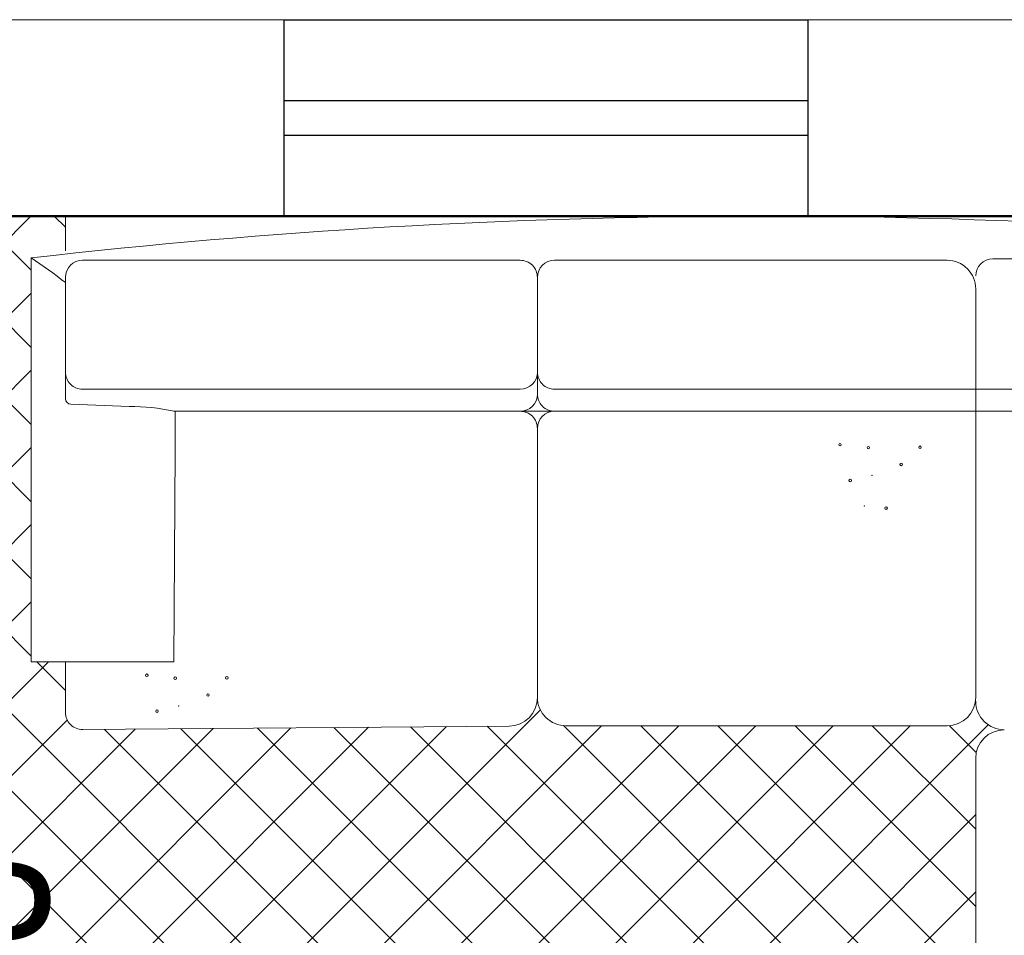
# Model space of a CAD drawing. Units: inches. Extents: x -466983 to 1020, y 324 to 318697.
# Tile 90 of 97: x 742 to 787, y 921 to 963. Entities that reach past the tile are written whole.
import ezdxf

# ---------------------------------------------------------------- set-up
doc = ezdxf.new("R2010")
doc.units = ezdxf.units.IN
doc.header["$MEASUREMENT"] = 0
for name, color, linetype, lineweight in [('A-ANNO-DIMS', 2, 'Continuous', 18), ('A-FLOR-PATT', 252, 'Continuous', 13), ('A-FURN', 8, 'Continuous', 18), ('A-GLAZ', 4, 'Continuous', 25), ('A-WALL', 7, 'Continuous', 50), ('L-SITE', 3, 'Continuous', 18)]:
    doc.layers.add(name, color=color, linetype=linetype, lineweight=lineweight)
doc.styles.get("Standard").update_dxf_attribs({"font": 'arial.ttf'})
doc.dimstyles.get("Standard").update_dxf_attribs({"dimtxt": 6, "dimasz": 4, "dimexe": 3, "dimexo": 3, "dimgap": 0.09, "dimtad": 0, "dimtih": 1, "dimtoh": 1, "dimdec": 1, "dimzin": 0, "dimdsep": 46, "dimlunit": 3, "dimtxsty": 'Standard', "dimcen": 0.09, "dimadec": 0, "dimazin": 0, "dimtfac": 1, "dimtdec": 1, "dimtofl": 0, "dimtmove": 0, "dimatfit": 3, "dimfxl": 1, "dimtolj": 1, "dimtzin": 0, "dimarcsym": 0})

# ---------------------------------------------------------------- blocks, each defined once
blk = doc.blocks.new('Window 2 ft')
for p, q in [((1298.676, 816.593), (1322.676, 816.593)), ((1298.676, 807.593), (1298.676, 816.593)), ((1322.676, 816.593), (1322.676, 807.593)), ((1298.676, 812.893), (1322.676, 812.893)), ((1322.676, 811.293), (1298.676, 811.293)), ((1322.676, 807.593), (1298.676, 807.593))]:
    blk.add_line(p, q)
blk = doc.blocks.new('L Shaped Sofa')
at = {"ltscale": 2}
for p, q in [((2438.01, 846.521), (2438.01, 834.581)), ((2471.772, 846.521), (2438.01, 846.521)), ((2438.01, 843.655), (2433.801, 843.655)), ((2460.02, 843.655), (2462.233, 843.655)), ((2470.142, 843.655), (2462.233, 843.655)), ((2475.263, 843.655), (2472.363, 843.655)), ((2475.263, 843.655), (2475.263, 821.686)), ((2459.543, 843.195), (2459.371, 838.325)), ((2432.653, 806.575), (2432.368, 842.211)), ((2460.8, 842.223), (2460.8, 821.686)), ((2471.575, 842.223), (2471.575, 821.686)), ((2455.692, 834.489), (2438.01, 834.581)), ((2458.96, 834.581), (2458.96, 805.639)), ((2455.692, 834.489), (2458.96, 834.489)), ((2460.8, 805.639), (2460.8, 821.686)), ((2471.575, 805.639), (2471.575, 821.686)), ((2475.263, 723.229), (2475.263, 821.686)), ((2458.96, 802.773), (2458.96, 805.639)), ((2435.071, 804.206), (2435.04, 804.206)), ((2457.527, 804.206), (2435.071, 804.206)), ((2457.527, 804.206), (2457.527, 804.206)), ((2462.233, 804.206), (2460.393, 804.206)), ((2470.142, 804.206), (2462.233, 804.206)), ((2458.96, 739.532), (2458.96, 802.773)), ((2460.8, 737.692), (2460.8, 802.773)), ((2471.575, 769.955), (2471.575, 802.773)), ((2432.683, 769.955), (2432.683, 801.818)), ((2429.959, 767.567), (2397.1, 767.567)), ((2469.187, 767.567), (2435.071, 767.567)), ((2471.701, 760.482), (2471.701, 766.134))]:
    blk.add_line(p, q, dxfattribs=at)
for centre, radius, start, end in [((2441.545, 866.112), 36.021, 321.43275, 327.0519), ((1939.075, 785.436), 536.188, 353.68225, 6.54157), ((2433.801, 842.223), 1.433, 90, 180.45787), ((2460.02, 843.178), 0.478, 90, 177.98163), ((2462.233, 842.223), 1.433, 90, 180), ((2470.142, 842.223), 1.433, 0, 90), ((2441.716, 838.368), 17.655, 347.61307, 359.85818), ((2436.906, 836.857), 0.106, 1.3946, 181.3946), ((2436.906, 836.857), 0.106, 181.3946, 1.3946), ((2433.902, 836.001), 0.106, 1.3946, 181.3946), ((2433.902, 836.001), 0.106, 181.3946, 1.3946), ((2436.655, 834.485), 0.106, 1.3946, 181.3946), ((2434.341, 834.182), 0.0177, 1.3946, 181.3946), ((2434.341, 834.182), 0.0177, 181.3946, 1.3946), ((2436.655, 834.485), 0.106, 181.3946, 1.3946), ((2435.251, 831.737), 0.106, 1.3946, 181.3946), ((2435.251, 831.737), 0.106, 181.3946, 1.3946), ((2436.686, 830.165), 0.106, 1.3946, 181.3946), ((2436.686, 830.165), 0.106, 181.3946, 1.3946), ((2435.04, 806.594), 2.388, 180.45787, 270), ((2457.527, 805.639), 1.433, 270, 0), ((2460.393, 805.639), 1.433, 180, 270), ((2462.233, 805.639), 1.433, 180, 270), ((2470.142, 805.639), 1.433, 270, 0), ((2435.071, 801.818), 2.388, 90, 180), ((2457.527, 802.773), 1.433, 0, 90), ((2460.393, 802.773), 1.433, 90, 180), ((2462.233, 802.773), 1.433, 90, 180), ((2470.142, 802.773), 1.433, 0, 90), ((2456.173, 778.913), 0.106, 1.3946, 181.3946), ((2456.173, 778.913), 0.106, 181.3946, 1.3946), ((2453.169, 778.058), 0.106, 1.3946, 181.3946), ((2453.169, 778.058), 0.106, 181.3946, 1.3946), ((2451.048, 776.875), 0.0177, 1.3946, 181.3946), ((2451.048, 776.875), 0.0177, 181.3946, 1.3946), ((2453.608, 776.239), 0.0177, 1.3946, 181.3946), ((2453.608, 776.239), 0.0177, 181.3946, 1.3946), ((2455.922, 776.541), 0.106, 1.3946, 181.3946), ((2455.922, 776.541), 0.106, 181.3946, 1.3946), ((2450.866, 775.061), 0.106, 1.3946, 181.3946), ((2450.866, 775.061), 0.106, 181.3946, 1.3946), ((2454.518, 773.793), 0.106, 1.3946, 181.3946), ((2454.518, 773.793), 0.106, 181.3946, 1.3946), ((2455.953, 772.221), 0.106, 1.3946, 181.3946), ((2455.953, 772.221), 0.106, 181.3946, 1.3946), ((2435.071, 769.955), 2.388, 180, 270), ((2469.187, 769.955), 2.388, 270, 0), ((2429.959, 765.179), 2.388, 0, 90), ((2434.735, 765.179), 2.388, 90, 180), ((2470.268, 766.134), 1.433, 0, 90)]:
    blk.add_arc(centre, radius, start, end, dxfattribs=at)
blk = doc.blocks.new('*D72')
at = {"layer": 'A-ANNO-DIMS', "color": 0, "lineweight": -2, "transparency": 16777216}
for p, q in [((739.215, 954.575), (728.974, 954.575)), ((731.974, 950.575), (731.974, 924.517)), ((731.974, 892.152), (731.974, 918.21)), ((739.215, 888.152), (728.974, 888.152))]:
    blk.add_line(p, q, dxfattribs=at)
at = {"layer": 'A-ANNO-DIMS', "color": 0, "transparency": 16777216}
for points in [[(731.307, 950.575), (732.641, 950.575), (731.974, 954.575)], [(731.307, 892.152), (732.641, 892.152), (731.974, 888.152)]]:
    blk.add_solid(points, dxfattribs=at)
at = {"layer": 'Defpoints', "color": 0, "transparency": 16777216}
for p in [(731.974, 954.575), (742.215, 954.575), (742.215, 888.152)]:
    blk.add_point(p, dxfattribs=at)
at = {"layer": 'A-ANNO-DIMS', "color": 0, "transparency": 16777216, "insert": (731.974, 921.363), "char_height": 6, "attachment_point": 5}
blk.add_mtext('\\A1;66 TYP.', dxfattribs=at)

msp = doc.modelspace()

# ---------------------------------------------------------------- hatches: boundary and pattern name
at = {"layer": 'A-FLOR-PATT', "transparency": 33554572}
h = msp.add_hatch(dxfattribs=at)
h.set_pattern_fill('ANSI37', color=256, scale=30)
h.set_pattern_definition([(45, (-1212.4137, -290.035), (-2.6516504, 2.6516504), []), (135, (-1212.4137, -290.035), (-2.6516504, -2.6516504), [])])
h.paths.add_polyline_path([(901.806, 1075.938), (900.614, 1075.938), (900.614, 1065.386), (899.391, 1065.386), (898.091, 1065.386), (892.836, 1058.71, -0.258377), (892.188, 1058.351), (879.985, 1058.351, -0.20177), (879.438, 1058.581), (874.081, 1065.386), (872.781, 1065.386), (871.558, 1065.386), (871.558, 1075.938), (813.806, 1075.938), (813.806, 1044.792), (832.395, 1044.792, -0.394795), (848.66, 1028.536), (848.66, 1009.938), (901.806, 1009.938), (901.806, 1015.938), (901.306, 1015.938), (871.306, 1015.938), (871.306, 1017.25), (871.334, 1017.25, -0.401453), (901.306, 1045.938), (901.806, 1045.938)])
edge = h.paths.add_edge_path(flags=16)
edge.add_line((847.773, 1068.949), (847.773, 1073.709))
edge.add_arc((849.227, 1073.709), 1.454, 90, 180, ccw=False)
edge.add_line((849.227, 1075.163), (864.492, 1075.163))
edge.add_arc((864.492, 1073.709), 1.454, 0, 90, ccw=False)
edge.add_line((865.946, 1073.709), (865.946, 1069.004))
edge.add_arc((832.645, 1068.976), 33.301, -20.6123, 0.0472, ccw=False)
edge.add_ellipse((856.859, 1058.48), major_axis=(0, 10.213), ratio=0.685919, start_angle=100.0088, end_angle=259.9912, ccw=False)
edge.add_arc((881.074, 1068.976), 33.301, 180.0472, 200.6123, ccw=False)
h.paths.add_polyline_path([(853.146, 1066.482), (853.146, 1066.453), (853.146, 1066.453, 0.433107), (852.917, 1066.685), (852.917, 1066.453), (853.146, 1066.453), (853.146, 1066.482), (853.088, 1066.612, 0.697939), (852.7, 1066.453), (852.7, 1066.453), (852.7, 1066.482), (852.917, 1067.001), (852.917, 1066.685, -0.396254)], flags=0)
h.paths.add_polyline_path([(861.019, 1066.482), (861.019, 1066.453), (861.019, 1066.453, 0.416404), (860.802, 1066.685), (860.802, 1066.453), (861.019, 1066.453), (861.019, 1066.482), (860.967, 1066.605, 0.713344), (860.573, 1066.453), (860.573, 1066.453), (860.573, 1066.482), (860.802, 1067.001), (860.802, 1066.685, -0.379973)], flags=0)
edge = h.paths.add_edge_path(flags=0)
edge.add_spline(control_points=[(861.13, 1065.785), (861.466, 1065.248), (861.613, 1065.016), (861.983, 1064.374), (862.192, 1063.944), (862.561, 1063.039), (862.721, 1062.563), (862.987, 1061.578), (863.092, 1061.069), (863.245, 1060.031), (863.293, 1059.503), (863.329, 1058.441), (863.318, 1057.908), (863.237, 1056.852), (863.166, 1056.329), (862.97, 1055.308), (862.843, 1054.81), (862.537, 1053.852), (862.357, 1053.393), (861.951, 1052.525), (861.725, 1052.117), (861.233, 1051.362), (860.967, 1051.016), (860.405, 1050.395), (860.108, 1050.12), (859.494, 1049.646), (859.176, 1049.448), (858.528, 1049.13), (858.197, 1049.011), (857.531, 1048.852), (857.196, 1048.812), (856.525, 1048.812), (856.189, 1048.852), (855.524, 1049.01), (855.193, 1049.129), (854.545, 1049.447), (854.227, 1049.645), (853.612, 1050.118), (853.316, 1050.393), (852.753, 1051.014), (852.487, 1051.36), (851.995, 1052.114), (851.769, 1052.523), (851.363, 1053.39), (851.183, 1053.85), (850.877, 1054.807), (850.75, 1055.305), (850.553, 1056.326), (850.483, 1056.849), (850.401, 1057.905), (850.39, 1058.438), (850.426, 1059.5), (850.473, 1060.028), (850.626, 1061.066), (850.732, 1061.575), (850.997, 1062.561), (851.157, 1063.036), (851.525, 1063.942), (851.734, 1064.371), (852.106, 1065.016), (852.254, 1065.25), (852.608, 1065.733)], knot_values=[3.915332, 3.915332, 3.915332, 3.915332, 4.013468, 4.013468, 4.175532, 4.175532, 4.337596, 4.337596, 4.49966, 4.49966, 4.661724, 4.661724, 4.823788, 4.823788, 4.985852, 4.985852, 5.147916, 5.147916, 5.30998, 5.30998, 5.472044, 5.472044, 5.634109, 5.634109, 5.796173, 5.796173, 5.958237, 5.958237, 6.120301, 6.120301, 6.282365, 6.282365, 6.444429, 6.444429, 6.606493, 6.606493, 6.768557, 6.768557, 6.930621, 6.930621, 7.092685, 7.092685, 7.254749, 7.254749, 7.416813, 7.416813, 7.578878, 7.578878, 7.740942, 7.740942, 7.903006, 7.903006, 8.06507, 8.06507, 8.227134, 8.227134, 8.389198, 8.389198, 8.551262, 8.551262, 8.65037, 8.65037, 8.65037, 8.65037], degree=3, periodic=0)
edge.add_line((852.642, 1065.785), (861.13, 1065.785))
edge = h.paths.add_edge_path(flags=0)
edge.add_ellipse((856.85, 1057.743), major_axis=(0, 7.792), ratio=0.687861, start_angle=0, end_angle=360)
h.paths.add_polyline_path([(848.863, 1069.389), (848.863, 1073.96, -0.414214), (849.954, 1075.051), (863.765, 1075.051, -0.414214), (864.856, 1073.96), (864.856, 1069.389, -0.388936), (864.524, 1069.027, -0.043561), (849.195, 1069.027, -0.388936)], flags=0)
h.paths.add_polyline_path([(853.101, 1068.112, -1), (852.677, 1068.112, -1)], flags=0)
edge = h.paths.add_edge_path(flags=0)
edge.add_ellipse((856.859, 1057.338), major_axis=(0, 2.207), ratio=0.657164, start_angle=0, end_angle=360)
h.paths.add_polyline_path([(861.041, 1068.112, -1), (860.618, 1068.112, -1)], flags=0)
edge = h.paths.add_edge_path()
edge.add_line((573.954, 1057.341), (573.954, 1075.938))
edge.add_line((573.954, 1075.938), (558.731, 1075.938))
edge.add_line((558.731, 1075.938), (558.731, 1065.386))
edge.add_line((558.731, 1065.386), (557.507, 1065.386))
edge.add_line((557.507, 1065.386), (556.207, 1065.386))
edge.add_line((556.207, 1065.386), (550.952, 1058.71))
edge.add_arc((550.304, 1059.116), 0.765, 270, 327.9483, ccw=False)
edge.add_line((550.304, 1058.351), (538.101, 1058.351))
edge.add_arc((538.101, 1059.116), 0.765, 224.3704, 270, ccw=False)
edge.add_line((537.555, 1058.581), (532.198, 1065.386))
edge.add_line((532.198, 1065.386), (530.898, 1065.386))
edge.add_line((530.898, 1065.386), (529.674, 1065.386))
edge.add_line((529.674, 1065.386), (529.674, 1075.938))
edge.add_line((529.674, 1075.938), (520.806, 1075.938))
edge.add_line((520.806, 1075.938), (520.806, 1045.938))
edge.add_line((520.806, 1045.938), (521.306, 1045.938))
edge.add_arc((521.306, 1015.938), 30, 2.5075, 90, ccw=False)
edge.add_line((551.277, 1017.25), (551.306, 1017.25))
edge.add_line((551.306, 1017.25), (551.306, 1015.938))
edge.add_line((551.306, 1015.938), (520.806, 1015.938))
edge.add_line((520.806, 1015.938), (520.806, 1009.938))
edge.add_line((520.806, 1009.938), (559.191, 1010.402))
edge.add_arc((559.191, 1011.856), 1.454, 180, 270, ccw=False)
edge.add_line((557.737, 1011.856), (557.737, 1016.561))
edge.add_arc((591.039, 1016.589), 33.301, 159.3877, 180.0472, ccw=False)
edge.add_ellipse((566.824, 1027.085), major_axis=(0, 10.213), ratio=0.685919, start_angle=280.0088, end_angle=439.9912, ccw=False)
edge.add_arc((542.609, 1016.589), 33.301, 0.0472, 20.6123, ccw=False)
edge.add_line((575.91, 1016.616), (575.91, 1011.856))
edge.add_arc((574.456, 1011.856), 1.454, -90, 0, ccw=False)
edge.add_line((574.456, 1010.402), (608.806, 1009.938))
edge.add_line((608.806, 1009.938), (608.806, 1041.086))
edge.add_line((608.806, 1041.086), (590.218, 1041.086))
edge.add_arc((590.775, 1057.907), 16.831, 181.9277, 268.1032, ccw=False)
edge = h.paths.add_edge_path()
edge.add_ellipse((494.244, 583.62), major_axis=(0, 10.213), ratio=0.685919, start_angle=280.0088, end_angle=439.9912, ccw=False)
edge.add_arc((470.03, 573.124), 33.301, 0.0472, 20.6123, ccw=False)
edge.add_line((503.331, 573.152), (503.331, 568.392))
edge.add_arc((501.877, 568.392), 1.454, -90, 0, ccw=False)
edge.add_line((501.877, 566.938), (539.806, 566.938))
edge.add_line((539.806, 566.938), (539.806, 572.938))
edge.add_line((539.806, 572.938), (539.306, 572.938))
edge.add_line((539.306, 572.938), (509.306, 572.938))
edge.add_line((509.306, 572.938), (509.306, 574.25))
edge.add_line((509.306, 574.25), (509.334, 574.25))
edge.add_arc((539.306, 572.938), 30, 90, 177.4925, ccw=False)
edge.add_line((539.306, 602.938), (539.806, 602.938))
edge.add_line((539.806, 602.938), (539.806, 626.938))
edge.add_line((539.806, 626.938), (531.772, 626.938))
edge.add_line((531.772, 626.938), (531.772, 616.386))
edge.add_line((531.772, 616.386), (530.548, 616.386))
edge.add_line((530.548, 616.386), (529.249, 616.386))
edge.add_line((529.249, 616.386), (523.711, 609.351))
edge.add_line((523.711, 609.351), (510.777, 609.351))
edge.add_line((510.777, 609.351), (505.239, 616.386))
edge.add_line((505.239, 616.386), (503.939, 616.386))
edge.add_line((503.939, 616.386), (502.715, 616.386))
edge.add_line((502.715, 616.386), (502.715, 626.938))
edge.add_line((502.715, 626.938), (481.698, 626.938))
edge.add_line((481.698, 626.938), (481.698, 610.995))
edge.add_arc((467.27, 611.473), 14.436, 271.9277, 358.1032, ccw=False)
edge.add_line((467.756, 597.045), (451.806, 597.045))
edge.add_line((451.806, 597.045), (451.806, 584.404))
edge.add_line((451.806, 584.404), (451.806, 566.938))
edge.add_line((451.806, 566.938), (486.612, 566.938))
edge.add_arc((486.612, 568.392), 1.454, 180, 270, ccw=False)
edge.add_line((485.158, 568.392), (485.158, 573.097))
edge.add_arc((518.459, 573.124), 33.301, 159.3877, 180.0472, ccw=False)
h.paths.add_polyline_path([(836.261, 1020.733), (879.89, 1020.733), (879.89, 1039.39), (836.261, 1039.39)], flags=25)
h.paths.add_polyline_path([(549.985, 1036.749), (593.614, 1036.749), (593.614, 1055.407), (549.985, 1055.407)], flags=24)
h.paths.add_polyline_path([(475.123, 595.596), (518.752, 595.596), (518.752, 614.253), (475.123, 614.253)], flags=24)
h = msp.add_hatch(dxfattribs=at)
h.set_pattern_fill('ANSI37', color=256, scale=20)
h.set_pattern_definition([(45, (-1212.4137, -290.035), (-1.767767, 1.767767), []), (135, (-1212.4137, -290.035), (-1.767767, -1.767767), [])])
h.paths.add_polyline_path([(809.806, 870.938), (809.806, 888.152), (806.998, 888.152), (802.662, 888.152), (789.383, 888.152), (786.285, 888.152, -0.414214), (785.499, 888.937), (785.499, 900.196), (785.499, 908.47, -0.414214), (786.808, 909.779, -0.414214), (785.499, 911.088), (785.499, 929.101, -0.414214), (786.808, 930.411, -0.414214), (785.499, 931.72), (785.499, 931.904, -0.414214), (784.19, 930.595), (766.722, 930.595, -0.412359), (765.413, 931.896, -0.413741), (764.115, 930.578), (744.578, 930.422, -0.416556), (743.786, 931.207), (743.786, 933.515), (742.215, 933.515), (742.215, 952.024, -0.001344), (743.786, 952.2), (743.786, 953.938), (678.592, 953.938), (678.592, 951.131), (678.592, 946.794), (678.592, 933.515), (678.592, 930.417, -0.414214), (677.806, 929.631), (666.548, 929.631), (658.274, 929.631, -0.414214), (656.965, 930.94, -0.414214), (655.656, 929.631), (637.642, 929.631, -0.414214), (636.333, 930.94, -0.414214), (635.024, 929.631), (634.839, 929.631, -0.414214), (636.149, 928.322), (636.149, 910.854, -0.412359), (634.848, 909.545, -0.413741), (636.165, 908.247), (636.321, 888.71, -0.416556), (635.536, 887.918), (633.228, 887.918), (633.228, 886.347), (614.719, 886.347, -0.001344), (614.544, 887.918), (612.806, 887.918), (612.806, 834.938), (612.806, 752.938), (612.806, 748.938), (612.806, 697.938), (654.806, 697.938), (654.806, 701.938), (715.806, 701.938), (715.806, 737.435), (774.292, 737.435), (774.292, 795.938), (809.806, 795.938)])
h.paths.add_polyline_path([(679.276, 849.576, 0.102523), (682.148, 849.261, -0.080461), (694.543, 849.773, -0.283899), (694.482, 849.008, 0.136605), (694.407, 848.81, -0.030441), (694.543, 846.893), (694.543, 842.62), (694.543, 838.347, -0.028219), (694.425, 836.568), (694.425, 836.568, 0.196187), (694.446, 836.271, -0.302897), (694.543, 835.467, -0.080461), (682.148, 835.979, 0.102523), (679.276, 835.664, -0.58611), (678.646, 836.017), (678.646, 849.223, -0.58611)], flags=16)
h.paths.add_polyline_path([(679.517, 848.651, 0.699597), (679.476, 848.634, 1.20716), (679.194, 848.742, 0.010621)], flags=0)
h.paths.add_polyline_path([(679.492, 836.561, -0.013798), (679.918, 836.659, -0.071703), (682.853, 837.143, -0.165743), (682.166, 839.101), (682.166, 842.609), (682.166, 846.06, -0.240616), (683.473, 848.677, -0.068263), (693.929, 849.008), (693.788, 848.708), (693.788, 849.023, 0.067332), (683.473, 848.677, 0.240616), (682.166, 846.06), (682.166, 842.609), (682.166, 839.101, 0.23459), (683.461, 836.551, 0.068093), (693.788, 836.195), (693.788, 836.51), (693.93, 836.21, -0.077215), (682.242, 836.782, 0.086627), (679.528, 836.57, -0.628402), (679.503, 836.573), (679.503, 836.607, 0.910458)], flags=0)
h.paths.add_polyline_path([(679.476, 848.636), (679.207, 848.647), (679.207, 836.572, 0.913566), (679.365, 836.586), (679.476, 836.582)], flags=0)
h.paths.add_polyline_path([(679.276, 829.86, 0.102523), (682.148, 829.546, -0.080461), (694.543, 830.057, -0.283899), (694.482, 829.293, 0.136605), (694.407, 829.095, -0.030441), (694.543, 827.178), (694.543, 822.904), (694.543, 818.631, -0.028219), (694.425, 816.853), (694.425, 816.853, 0.196187), (694.446, 816.556, -0.302897), (694.543, 815.752, -0.080461), (682.148, 816.263, 0.102523), (679.276, 815.949, -0.58611), (678.646, 816.302), (678.646, 829.507, -0.58611)], flags=16)
h.paths.add_polyline_path([(679.517, 828.936, 0.699597), (679.476, 828.919, 1.20716), (679.194, 829.027, 0.010621)], flags=0)
h.paths.add_polyline_path([(679.492, 816.846, -0.013798), (679.918, 816.944, -0.071703), (682.853, 817.428, -0.165743), (682.166, 819.385), (682.166, 822.894), (682.166, 826.345, -0.240616), (683.473, 828.961, -0.068263), (693.929, 829.293), (693.788, 828.993), (693.788, 829.308, 0.067332), (683.473, 828.961, 0.240616), (682.166, 826.345), (682.166, 822.894), (682.166, 819.385, 0.23459), (683.461, 816.836, 0.068093), (693.788, 816.48), (693.788, 816.795), (693.93, 816.495, -0.077215), (682.242, 817.066, 0.086627), (679.528, 816.855, -0.628402), (679.503, 816.858), (679.503, 816.892, 0.910458)], flags=0)
h.paths.add_polyline_path([(679.476, 828.921), (679.207, 828.932), (679.207, 816.857, 0.913566), (679.365, 816.871), (679.476, 816.867)], flags=0)
h.paths.add_polyline_path([(679.276, 810.145, 0.102523), (682.148, 809.83, -0.080461), (694.543, 810.342, -0.3023), (694.447, 809.539, 0.10023), (694.406, 809.388, -0.03057), (694.543, 807.462), (694.543, 803.189), (694.543, 798.916, -0.03057), (694.406, 796.991, 0.10023), (694.447, 796.839, -0.3023), (694.543, 796.036, -0.080461), (682.148, 796.548, 0.102523), (679.276, 796.233, -0.58611), (678.646, 796.586), (678.646, 809.792, -0.58611)], flags=16)
h.paths.add_polyline_path([(679.517, 809.242, 0.699597), (679.476, 809.224, 1.20716), (679.194, 809.332, 0.010621)], flags=0)
h.paths.add_polyline_path([(679.492, 797.151, -0.013798), (679.918, 797.25, -0.071703), (682.853, 797.734, -0.165743), (682.166, 799.691), (682.166, 803.2), (682.166, 806.65, -0.239349), (683.461, 809.258, -0.072465), (694.447, 809.541, 0.197932), (694.425, 809.241), (693.788, 809.299), (693.788, 809.614, 0.068093), (683.461, 809.258, 0.239349), (682.166, 806.65), (682.166, 803.2), (682.166, 799.691, 0.235854), (683.473, 797.132, 0.067332), (693.788, 796.786), (693.788, 797.101), (694.425, 797.159, 0.197932), (694.447, 796.859, -0.080419), (682.156, 797.379, 0.083867), (679.528, 797.16, -0.628402), (679.503, 797.164), (679.503, 797.197, 0.910458)], flags=0)
h.paths.add_polyline_path([(679.207, 809.237), (679.207, 797.162, 0.913566), (679.365, 797.176), (679.476, 797.173), (679.476, 809.227)], flags=0)
h.paths.add_polyline_path([(695.364, 853.299), (728.223, 853.299), (728.223, 771.152), (695.364, 771.152)], flags=16)
h.paths.add_polyline_path([(696.021, 852.642), (727.566, 852.642), (727.566, 771.809), (696.021, 771.809)], flags=0)
h.paths.add_polyline_path([(679.276, 788.787, 0.102523), (682.148, 788.472, -0.080461), (694.543, 788.984, -0.3023), (694.447, 788.181, 0.10023), (694.406, 788.03, -0.03057), (694.543, 786.104), (694.543, 781.831), (694.543, 777.558, -0.03057), (694.406, 775.632, 0.10023), (694.447, 775.481, -0.3023), (694.543, 774.678, -0.080461), (682.148, 775.19, 0.102523), (679.276, 774.875, -0.58611), (678.646, 775.228), (678.646, 788.434, -0.58611)], flags=16)
h.paths.add_polyline_path([(679.517, 787.883, 0.699597), (679.476, 787.866, 1.20716), (679.194, 787.974, 0.010621)], flags=0)
h.paths.add_polyline_path([(679.492, 775.793, -0.013798), (679.918, 775.891, -0.071703), (682.853, 776.375, -0.165743), (682.166, 778.333), (682.166, 781.841), (682.166, 785.292, -0.239349), (683.461, 787.899, -0.072465), (694.447, 788.182, 0.197932), (694.425, 787.882), (693.788, 787.94), (693.788, 788.255, 0.068093), (683.461, 787.899, 0.239349), (682.166, 785.292), (682.166, 781.841), (682.166, 778.333, 0.235854), (683.473, 775.774, 0.067332), (693.788, 775.428), (693.788, 775.742), (694.425, 775.8, 0.197932), (694.447, 775.5, -0.080419), (682.156, 776.021, 0.083867), (679.528, 775.802, -0.628402), (679.503, 775.805), (679.503, 775.839, 0.910458)], flags=0)
h.paths.add_polyline_path([(679.207, 787.879), (679.207, 775.804, 0.913566), (679.365, 775.818), (679.476, 775.814), (679.476, 787.868)], flags=0)
h.paths.add_polyline_path([(704.641, 854.12, -0.080461), (705.153, 866.516, 0.102523), (704.838, 869.387, -0.58611), (705.191, 870.017), (718.397, 870.017, -0.58611), (718.75, 869.387, 0.102523), (718.435, 866.516, -0.080461), (718.946, 854.12, -0.3023), (718.144, 854.217, 0.10023), (717.992, 854.257, -0.03057), (716.067, 854.12), (711.794, 854.12), (707.521, 854.12, -0.03057), (705.595, 854.257, 0.10023), (705.444, 854.217, -0.3023)], flags=16)
h.paths.add_polyline_path([(717.846, 869.146, 0.699597), (717.829, 869.187, 1.20716), (717.937, 869.47, 0.010621)], flags=0)
h.paths.add_polyline_path([(705.463, 854.216, -0.080419), (705.984, 866.507, 0.083867), (705.765, 869.135, -0.628402), (705.768, 869.16), (705.802, 869.16, 0.910458), (705.756, 869.171, -0.013798), (705.854, 868.745, -0.071703), (706.338, 865.81, -0.165743), (708.295, 866.497), (711.804, 866.497), (715.255, 866.497, -0.239349), (717.862, 865.202, -0.072465), (718.145, 854.216, 0.197932), (717.845, 854.238), (717.903, 854.876), (718.218, 854.876, 0.068093), (717.862, 865.202, 0.239349), (715.255, 866.497), (711.804, 866.497), (708.295, 866.497, 0.235854), (705.737, 865.19, 0.067332), (705.391, 854.876), (705.705, 854.876), (705.763, 854.238, 0.197932)], flags=16)
h.paths.add_polyline_path([(705.766, 869.456, 0.913566), (705.781, 869.299), (705.777, 869.187), (717.831, 869.187), (717.842, 869.456)], flags=0)
h.paths.add_polyline_path([(729.045, 842.62), (729.045, 846.893, -0.03057), (729.182, 848.818, 0.10023), (729.141, 848.97, -0.3023), (729.045, 849.773, -0.080461), (741.44, 849.261, 0.102523), (744.311, 849.576, -0.58611), (744.942, 849.223), (744.942, 836.017, -0.58611), (744.311, 835.664, 0.102523), (741.44, 835.979, -0.080461), (729.045, 835.467, -0.3023), (729.141, 836.27, 0.10023), (729.182, 836.421, -0.03057), (729.045, 838.347)], flags=16)
h.paths.add_polyline_path([(744.111, 836.585, 1.20716), (744.394, 836.477, 0.010621), (744.07, 836.567, 0.699597)], flags=0)
h.paths.add_polyline_path([(729.141, 836.268, 0.197932), (729.162, 836.568), (729.8, 836.51), (729.8, 836.195, 0.068093), (740.126, 836.551, 0.239349), (741.421, 839.159), (741.421, 842.609), (741.421, 846.118, 0.235854), (740.114, 848.677, 0.067332), (729.8, 849.023), (729.8, 848.708), (729.162, 848.65, 0.197932), (729.141, 848.95, -0.080419), (741.432, 848.43, 0.083867), (744.059, 848.649, -0.628402), (744.085, 848.645), (744.085, 848.612, 0.910458), (744.095, 848.658, -0.013798), (743.67, 848.559, -0.071703), (740.734, 848.075, -0.165743), (741.421, 846.118), (741.421, 842.609), (741.421, 839.159, -0.239349), (740.126, 836.551, -0.072465)], flags=0)
h.paths.add_polyline_path([(729.045, 830.057, -0.080461), (741.44, 829.546, 0.102523), (744.311, 829.86, -0.58611), (744.942, 829.507), (744.942, 816.302, -0.58611), (744.311, 815.949, 0.102523), (741.44, 816.263, -0.080461), (729.045, 815.752, -0.3023), (729.141, 816.554, 0.10023), (729.182, 816.706, -0.03057), (729.045, 818.631), (729.045, 822.904), (729.045, 827.178, -0.03057), (729.182, 829.103, 0.10023), (729.141, 829.255, -0.3023)], flags=16)
h.paths.add_polyline_path([(744.111, 816.869, 1.20716), (744.394, 816.761, 0.010621), (744.07, 816.852, 0.699597)], flags=0)
h.paths.add_polyline_path([(729.141, 829.235, -0.080419), (741.432, 828.714, 0.083867), (744.059, 828.933, -0.628402), (744.085, 828.93), (744.085, 828.896, 0.910458), (744.095, 828.943, -0.013798), (743.67, 828.844, -0.071703), (740.734, 828.36, -0.165743), (741.421, 826.403), (741.421, 822.894), (741.421, 819.443, -0.239349), (740.126, 816.836, -0.072465), (729.141, 816.553, 0.197932), (729.162, 816.853), (729.8, 816.795), (729.8, 816.48, 0.068093), (740.126, 816.836, 0.239349), (741.421, 819.443), (741.421, 822.894), (741.421, 826.403, 0.235854), (740.114, 828.961, 0.067332), (729.8, 829.308), (729.8, 828.993), (729.162, 828.935, 0.197932)], flags=16)
h.paths.add_polyline_path([(729.045, 810.342, -0.080461), (741.44, 809.83, 0.102523), (744.311, 810.145, -0.58611), (744.942, 809.792), (744.942, 796.586, -0.58611), (744.311, 796.233, 0.102523), (741.44, 796.548, -0.080461), (729.045, 796.036, -0.283899), (729.105, 796.801, 0.136605), (729.181, 796.999, -0.030441), (729.045, 798.916), (729.045, 803.189), (729.045, 807.462, -0.028219), (729.163, 809.241), (729.162, 809.241, 0.196187), (729.142, 809.538, -0.302897)], flags=16)
h.paths.add_polyline_path([(744.111, 797.175, 1.20716), (744.394, 797.067, 0.010621), (744.07, 797.158, 0.699597)], flags=0)
h.paths.add_polyline_path([(741.345, 809.027, 0.086627), (744.059, 809.239, -0.628402), (744.085, 809.235), (744.085, 809.202, 0.910458), (744.095, 809.248, -0.013798), (743.67, 809.15, -0.071703), (740.734, 808.666, -0.165743), (741.421, 806.708), (741.421, 803.2), (741.421, 799.749, -0.240616), (740.114, 797.132, -0.068263), (729.658, 796.801), (729.8, 797.101), (729.8, 796.786, 0.067332), (740.114, 797.132, 0.240616), (741.421, 799.749), (741.421, 803.2), (741.421, 806.708, 0.23459), (740.126, 809.258, 0.068093), (729.8, 809.614), (729.8, 809.299), (729.658, 809.599, -0.077215)], flags=0)
h.paths.add_polyline_path([(704.641, 770.33, -0.283899), (705.405, 770.27, 0.136605), (705.603, 770.194, -0.030441), (707.521, 770.33), (711.794, 770.33), (716.067, 770.33, -0.028219), (717.845, 770.212), (717.845, 770.213, 0.196187), (718.143, 770.233, -0.302897), (718.946, 770.33, -0.080461), (718.435, 757.935, 0.102523), (718.75, 755.064, -0.58611), (718.397, 754.433), (705.191, 754.433, -0.58611), (704.838, 755.064, 0.102523), (705.153, 757.935, -0.080461)], flags=16)
h.paths.add_polyline_path([(705.762, 755.305, 0.699597), (705.779, 755.264, 1.20716), (705.671, 754.981, 0.010621)], flags=0)
h.paths.add_polyline_path([(705.405, 769.717), (705.705, 769.575), (705.391, 769.575, 0.067332), (705.737, 759.261, 0.240616), (708.353, 757.954), (711.804, 757.954), (715.313, 757.954, 0.23459), (717.862, 759.249, 0.068093), (718.218, 769.575), (717.903, 769.575), (718.203, 769.717, -0.077215), (717.632, 758.03, 0.086627), (717.843, 755.316, -0.628402), (717.84, 755.29), (717.806, 755.29, 0.910458), (717.853, 755.28, -0.013798), (717.754, 755.705, -0.071703), (717.27, 758.641, -0.165743), (715.313, 757.954), (711.804, 757.954), (708.353, 757.954, -0.240616), (705.737, 759.261, -0.068263)], flags=0)
h.paths.add_polyline_path([(729.045, 788.984, -0.080461), (741.44, 788.472, 0.102523), (744.311, 788.787, -0.58611), (744.942, 788.434), (744.942, 775.228, -0.58611), (744.311, 774.875, 0.102523), (741.44, 775.19, -0.080461), (729.045, 774.678, -0.283899), (729.105, 775.443, 0.136605), (729.181, 775.64, -0.030441), (729.045, 777.558), (729.045, 781.831), (729.045, 786.104, -0.028219), (729.163, 787.882), (729.162, 787.882, 0.196187), (729.142, 788.18, -0.302897)], flags=16)
h.paths.add_polyline_path([(744.111, 775.817, 1.20716), (744.394, 775.709, 0.010621), (744.07, 775.799, 0.699597)], flags=0)
h.paths.add_polyline_path([(741.345, 787.669, 0.086627), (744.059, 787.881, -0.628402), (744.085, 787.877), (744.085, 787.844, 0.910458), (744.095, 787.89, -0.013798), (743.67, 787.791, -0.071703), (740.734, 787.307, -0.165743), (741.421, 785.35), (741.421, 781.841), (741.421, 778.39, -0.240616), (740.114, 775.774, -0.068263), (729.658, 775.443), (729.8, 775.742), (729.8, 775.428, 0.067332), (740.114, 775.774, 0.240616), (741.421, 778.39), (741.421, 781.841), (741.421, 785.35, 0.23459), (740.126, 787.899, 0.068093), (729.8, 788.255), (729.8, 787.94), (729.658, 788.241, -0.077215)], flags=0)
h.paths.add_polyline_path([(744.111, 848.636), (744.111, 836.582), (744.381, 836.572), (744.381, 848.647, 0.913566), (744.223, 848.633)], flags=0)
h.paths.add_polyline_path([(744.223, 828.917), (744.111, 828.921), (744.111, 816.867), (744.381, 816.857), (744.381, 828.932, 0.913566)], flags=0)
h.paths.add_polyline_path([(717.831, 755.264), (705.777, 755.264), (705.766, 754.994), (717.842, 754.994, 0.913566), (717.827, 755.152)], flags=0)
h.paths.add_polyline_path([(744.223, 809.223), (744.111, 809.227), (744.111, 797.173), (744.381, 797.162), (744.381, 809.237, 0.913566)], flags=0)
h.paths.add_polyline_path([(744.111, 787.868), (744.111, 775.814), (744.381, 775.804), (744.381, 787.879, 0.913566), (744.223, 787.865)], flags=0)
h.paths.add_polyline_path([(678.877, 877.123), (737.613, 877.123), (737.613, 899.512), (678.877, 899.512)], flags=24)

# ---------------------------------------------------------------- linework, layer by layer
at = {"layer": 'A-WALL'}
msp.add_line((740.215, 953.938), (809.806, 953.938), dxfattribs=at)
at = {"layer": 'L-SITE'}
msp.add_line((617.806, 962.938), (804.806, 962.938), dxfattribs=at)

# ---------------------------------------------------------------- block references
at = {"layer": 'A-FURN', "xscale": 0.5482153745360612, "yscale": 0.5482153745360612, "zscale": 0.5482153745360612, "rotation": 89.99999999999999}
msp.add_blockref('L Shaped Sofa', (1206.291, -403.039), dxfattribs=at)
at = {"layer": 'A-GLAZ', "rotation": 180}
msp.add_blockref('Window 2 ft', (2076.482, 1770.531), dxfattribs=at)

# ---------------------------------------------------------------- dimensions: what is measured, and where the dimension line sits
at = {"layer": 'A-ANNO-DIMS'}
dim = msp.add_linear_dim(base=(731.974, 954.575), p1=(742.215, 888.152), p2=(742.215, 954.575), angle=90, text='<> TYP.', dimstyle='Standard', override={"dimdec": 0, "dimlfac": 1, "dimrnd": 0, "dimzin": 0, "dimdsep": 46, "dimlunit": 2}, dxfattribs=at)
dim.commit()
dim.dimension.update_dxf_attribs({"geometry": '*D72', "text_midpoint": (731.974, 921.363)})

doc.saveas('drawing.dxf')
